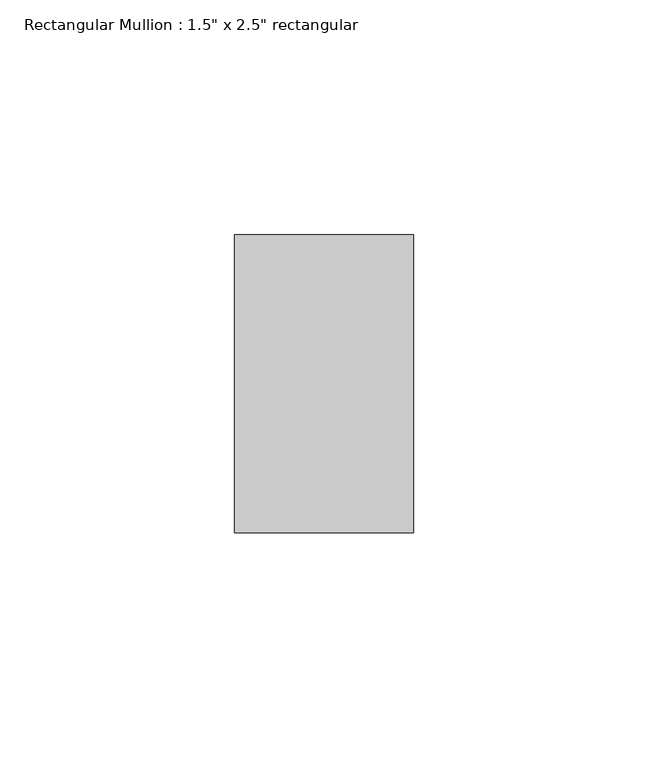
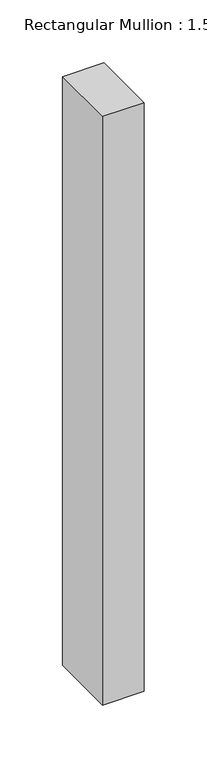
"""IFC4 building model written with IfcOpenShell, lengths in millimetres: member geometry."""

from ifc_helpers import new_model, si_unit, frame, origin, place, context, project, spatial, polyline, outline, extrude, source, transform, mapped, element, save


def member_b8e7570c(model_context):
    return source(origin(), model_context, "Body", "SweptSolid", [
        extrude(outline(polyline([(19.05, 31.75), (19.05, -31.75), (-19.05, -31.75), (-19.05, 31.75), (19.05, 31.75)])), frame((0.0, 0.0, -571.5), z_axis=(0.0, 0.0, 1.0), x_axis=(1.0, 0.0, 0.0)), (0.0, 0.0, 1.0), 571.5),
    ])


if __name__ == "__main__":
    model = new_model("IFC4")
    model_context = context("Model", 3, world=origin())
    ifc_project = project(units=[si_unit("LENGTHUNIT", "METRE", prefix="MILLI")], contexts=[model_context])
    site = spatial("IfcSite", under=ifc_project)
    building = spatial("IfcBuilding", under=site)
    placement = place(None, origin())
    member_shape = member_b8e7570c(model_context)
    element("IfcMember", 1, ObjectType="Rectangular Mullion : 1.5\" x 2.5\" rectangular", at=placement, inside=building, context=model_context, shape_type="MappedRepresentation", body=[
        mapped(member_shape, transform((0.0, 0.0, 0.0), x_axis=(1.0, 0.0, 0.0), y_axis=(0.0, 1.0, 0.0), z_axis=(0.0, 0.0, 1.0))),
    ])
    save(model, "model.ifc")

# Revit data of these elements
# Type "Rectangular Mullion : 1.5\" x 2.5\" rectangular"
#   built-in parameter 1007304 = 0.208333 (stored number, unit not read)
#   built-in parameter 1007301 = 0.0625 (stored number, unit not read)
#   built-in parameter 1007300 = 0.0625 (stored number, unit not read)
# Element 1 (IfcMember, "Rectangular Mullion : 1.5\" x 2.5\" rectangular")
#   Materials on its faces: "Aluminum"
# Materials
#   "Aluminum": class "Metal", colour RGB 247 247 247, transparency 0, Description = "Aluminum 6061", Cost = 0
